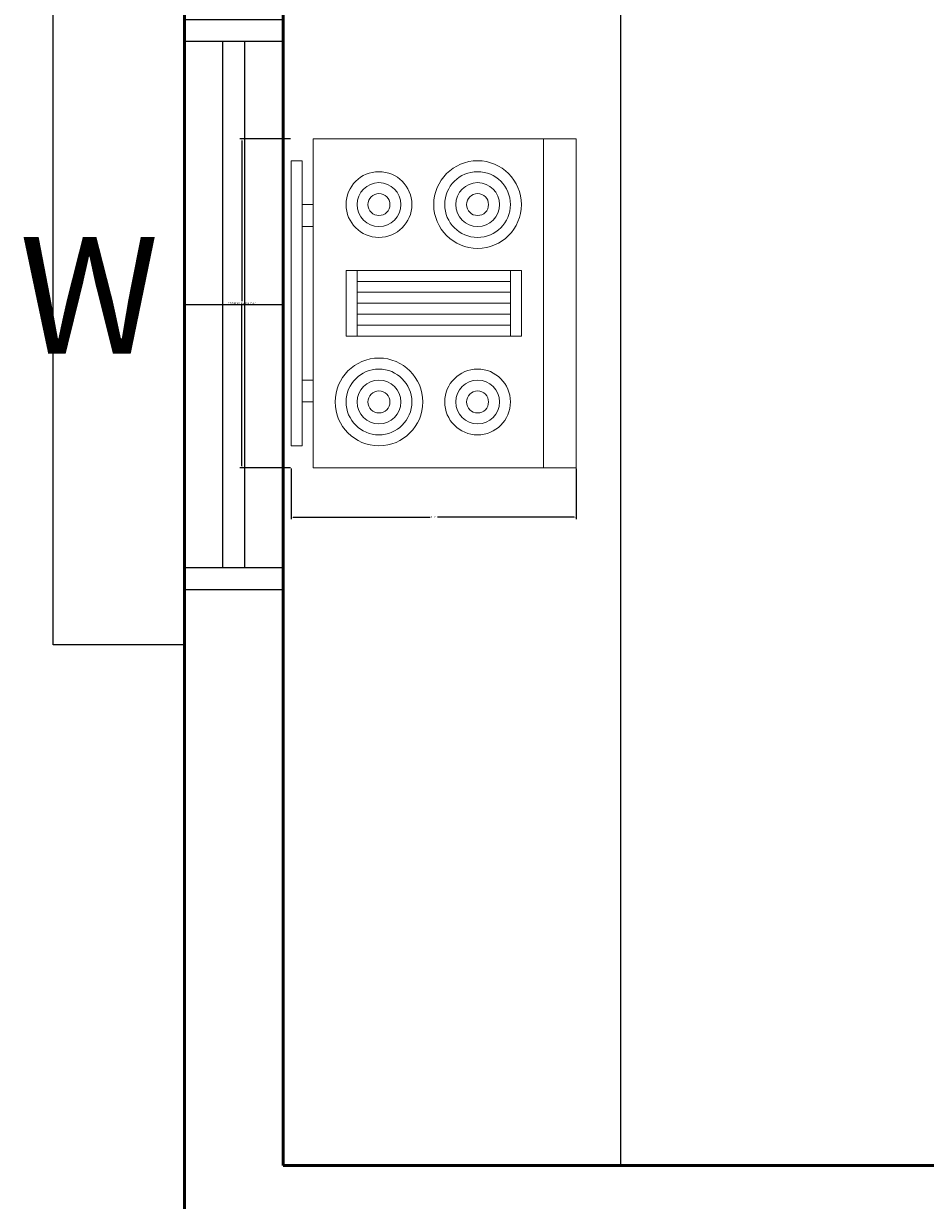
# Model space of a CAD drawing. Units: inches. Extents: x -105 to 1196, y -792 to 119.
# Tile 4 of 23: x -60 to 22, y -285 to -178. Entities that reach past the tile are written whole.
import ezdxf

# ---------------------------------------------------------------- set-up
doc = ezdxf.new("R2010")
doc.units = ezdxf.units.IN
doc.header["$MEASUREMENT"] = 0
for name, color, linetype, lineweight in [('A-ANNO-DIMS', 2, 'Continuous', 18), ('A-ANNO-TEXT', 7, 'Continuous', 25), ('A-FLOR-FIXT', 8, 'Continuous', 18), ('A-GLAZ', 4, 'Continuous', 25), ('A-WALL', 3, 'Continuous', 50)]:
    doc.layers.add(name, color=color, linetype=linetype, lineweight=lineweight)
doc.styles.get("Standard").update_dxf_attribs({"font": 'arial.ttf'})
doc.dimstyles.get("Standard").update_dxf_attribs({"dimtxt": 0.18, "dimasz": 0.18, "dimexe": 0.18, "dimexo": 0.0625, "dimgap": 0.09, "dimtad": 0, "dimtih": 1, "dimtoh": 1, "dimdec": 1, "dimzin": 0, "dimdsep": 46, "dimlunit": 4, "dimtxsty": 'Standard', "dimcen": 0.09, "dimadec": 0, "dimazin": 0, "dimtfac": 1, "dimtdec": 1, "dimtofl": 0, "dimtmove": 0, "dimatfit": 3, "dimfxl": 1, "dimtolj": 1, "dimtzin": 0, "dimarcsym": 0})

# ---------------------------------------------------------------- blocks, each defined once
blk = doc.blocks.new('Range-Oven - 30 in top')
for p, q in [((0, -3), (30, -3)), ((12, -6), (18, -6)), ((13, -20), (13, -6)), ((14, -6), (14, -20)), ((15, -20), (15, -6)), ((16, -6), (16, -20)), ((17, -20), (17, -6)), ((18, -20), (12, -20)), ((6, -24), (6, -25)), ((8, -25), (8, -24)), ((22, -25), (22, -24)), ((24, -24), (24, -25))]:
    blk.add_line(p, q)
for points in [[(0, -24), (0, 0), (30, 0), (30, -24)], [(12, -21), (12, -5), (18, -5), (18, -21)], [(2, -26), (2, -25), (28, -25), (28, -26)]]:
    blk.add_lwpolyline(points, close=True)
for centre, radius in [((6, -9), 4), ((6, -9), 3), ((24, -9), 3), ((6, -9), 2), ((24, -9), 2), ((6, -9), 1), ((24, -9), 1), ((6, -18), 3), ((24, -18), 4), ((24, -18), 3), ((6, -18), 2), ((24, -18), 2), ((6, -18), 1), ((24, -18), 1)]:
    blk.add_circle(centre, radius)
blk = doc.blocks.new('WIN-1200')
at = {"ltscale": 2}
for p, q in [((12, 62), (0, 62)), ((0, 0), (0, 62)), ((12, 57), (12, 62)), ((12, 5), (12, 0)), ((12, 0), (0, 0))]:
    blk.add_line(p, q, dxfattribs=at)
for p, q in [((21, 57), (12, 57)), ((21, 5), (12, 5))]:
    blk.add_line(p, q)
blk = doc.blocks.new('*D85')
at = {"layer": 'A-ANNO-DIMS', "color": 0, "lineweight": -2, "transparency": 16777216}
for p, q in [((-35.59, -188.59), (-40.2, -188.59)), ((-40.02, -188.77), (-40.02, -203.4)), ((-40.02, -218.41), (-40.02, -203.77)), ((-35.59, -218.59), (-40.2, -218.59))]:
    blk.add_line(p, q, dxfattribs=at)
at = {"layer": 'A-ANNO-DIMS', "color": 0, "transparency": 16777216}
for points in [[(-40.05, -188.77), (-39.99, -188.77), (-40.02, -188.59)], [(-40.05, -218.41), (-39.99, -218.41), (-40.02, -218.59)]]:
    blk.add_solid(points, dxfattribs=at)
at = {"layer": 'Defpoints', "color": 0, "transparency": 16777216}
for p in [(-35.52, -188.59), (-40.02, -218.59), (-35.52, -218.59)]:
    blk.add_point(p, dxfattribs=at)
at = {"layer": 'A-ANNO-DIMS', "color": 0, "transparency": 16777216, "insert": (-40.02, -203.59), "char_height": 0.18, "attachment_point": 5}
blk.add_mtext('\\A1;COOKING RANGE 2\'-6"', dxfattribs=at)
blk = doc.blocks.new('*D86')
at = {"layer": 'A-ANNO-DIMS', "color": 0, "lineweight": -2, "transparency": 16777216}
for p, q in [((-35.52, -218.65), (-35.52, -223.27)), ((-9.52, -218.65), (-9.52, -223.27)), ((-35.34, -223.09), (-22.85, -223.09)), ((-9.7, -223.09), (-22.19, -223.09))]:
    blk.add_line(p, q, dxfattribs=at)
at = {"layer": 'A-ANNO-DIMS', "color": 0, "transparency": 16777216}
for points in [[(-35.34, -223.06), (-35.34, -223.12), (-35.52, -223.09)], [(-9.7, -223.06), (-9.7, -223.12), (-9.52, -223.09)]]:
    blk.add_solid(points, dxfattribs=at)
at = {"layer": 'Defpoints', "color": 0, "transparency": 16777216}
for p in [(-35.52, -218.59), (-9.52, -218.59), (-9.52, -223.09)]:
    blk.add_point(p, dxfattribs=at)
at = {"layer": 'A-ANNO-DIMS', "color": 0, "transparency": 16777216, "insert": (-22.52, -223.09), "char_height": 0.18, "attachment_point": 5}
blk.add_mtext('\\A1;2\'-2"', dxfattribs=at)

msp = doc.modelspace()

# ---------------------------------------------------------------- linework, layer by layer
at = {"layer": 'A-GLAZ'}
for p, q in [((-5.49, -149.97), (-5.49, -282.23)), ((-36.26, -179.73), (-45.26, -179.73)), ((-41.76, -227.73), (-41.76, -179.73)), ((-39.76, -227.73), (-39.76, -179.73)), ((-36.26, -203.73), (-45.26, -203.73)), ((-36.26, -227.73), (-45.26, -227.73))]:
    msp.add_line(p, q, dxfattribs=at)
at = {"layer": 'A-WALL'}
for p, q in [((-45.26, -125.23), (-45.26, -291.23)), ((-36.26, -125.23), (-36.26, -282.23)), ((-36.26, -282.23), (129.74, -282.23))]:
    msp.add_line(p, q, dxfattribs=at)

# ---------------------------------------------------------------- block references
at = {"layer": 'A-FLOR-FIXT', "rotation": 270}
msp.add_blockref('Range-Oven - 30 in top', (-9.52, -188.59), dxfattribs=at)
at = {"layer": 'A-GLAZ'}
msp.add_blockref('WIN-1200', (-57.26, -234.73), dxfattribs=at)

# ---------------------------------------------------------------- texts
at = {"layer": 'A-ANNO-TEXT'}
msp.add_text('W', height=10.64, dxfattribs=at).set_placement((-60.33, -208.18))

# ---------------------------------------------------------------- dimensions: what is measured, and where the dimension line sits
at = {"layer": 'A-ANNO-DIMS'}
dim = msp.add_linear_dim(base=(-40.02, -218.59), p1=(-35.52, -188.59), p2=(-35.52, -218.59), angle=270, text='COOKING RANGE <>', dimstyle='Standard', override={"dimdec": 1, "dimlfac": 1, "dimrnd": 0, "dimzin": 1, "dimdsep": 46, "dimlunit": 4, "dimfrac": 2}, dxfattribs=at)
dim.commit()
dim.dimension.update_dxf_attribs({"geometry": '*D85', "text_midpoint": (-40.02, -203.59)})
dim = msp.add_linear_dim(base=(-9.52, -223.09), p1=(-35.52, -218.59), p2=(-9.52, -218.59), dimstyle='Standard', override={"dimdec": 1, "dimlfac": 1, "dimrnd": 0, "dimzin": 1, "dimdsep": 46, "dimlunit": 4, "dimfrac": 2}, dxfattribs=at)
dim.commit()
dim.dimension.update_dxf_attribs({"geometry": '*D86', "text_midpoint": (-22.52, -223.09)})

doc.saveas('drawing.dxf')
